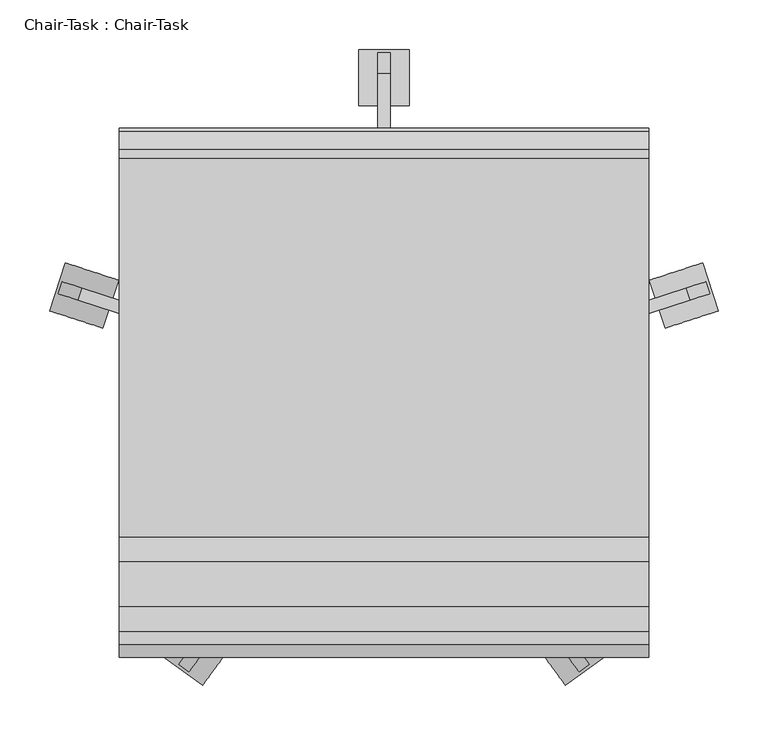
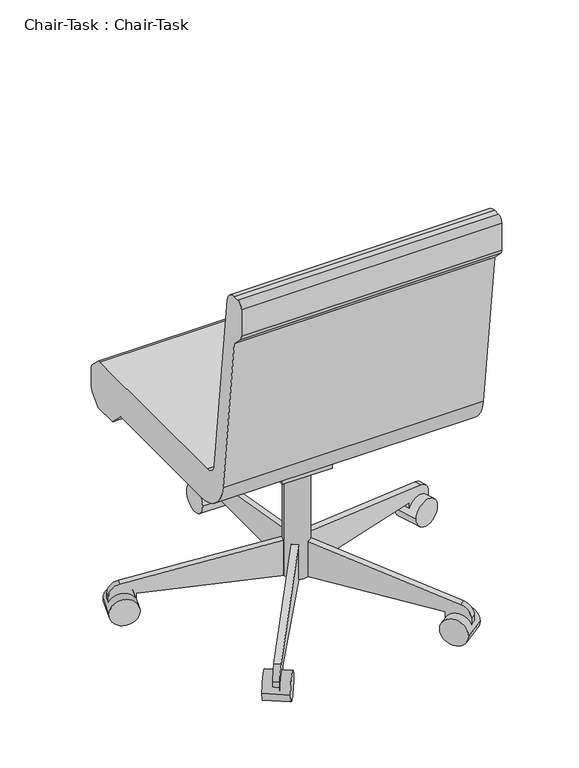
"""IFC4 building model written with IfcOpenShell, lengths in millimetres: furniture geometry, Chair-Task : Chair-Task."""

from ifc_helpers import new_model, si_unit, point, frame, frame_2d, origin, place, context, project, spatial, polyline, circle_curve, trimmed, segment, composite_curve, outline, extrude, source, transform, mapped, element, save


def chair_task_chair_task_b7f3823b(model_context):
    return source(origin(), model_context, "Body", "SweptSolid", [
        extrude(outline(composite_curve([segment(trimmed(circle_curve(frame_2d((140.9908197, 18.9459016)), 25.4), [point((115.5908197, 18.9459016))], [point((166.3908197, 18.9459016))], False, "CARTESIAN"), True, "CONTINUOUS"), segment(trimmed(circle_curve(frame_2d((140.9908197, 18.9459016)), 25.4), [point((166.3908197, 18.9459016))], [point((115.5908197, 18.9459016))], False, "CARTESIAN"), True, "CONTINUOUS")], self_intersect=False)), frame((0.0, 0.0, 53.5835944), z_axis=(0.0, 0.0, 1.0), x_axis=(1.0, 0.0, 0.0)), (0.0, 0.0, 1.0), 330.5914056),
        extrude(outline(composite_curve([segment(trimmed(circle_curve(frame_2d((0.0, -28.2002727)), 28.2002727), [point((0.0, -56.4005455))], [point((0.0, 0.0))], False, "CARTESIAN"), True, "CONTINUOUS"), segment(trimmed(circle_curve(frame_2d((0.0, -28.2002727)), 28.2002727), [point((0.0, 0.0))], [point((0.0, -56.4005455))], False, "CARTESIAN"), True, "CONTINUOUS")], self_intersect=False)), frame((477.6203484, 101.6163254, 28.1835944), z_axis=(-0.3090169943749423, 0.9510565162951553, 0.0), x_axis=(0.0, 0.0, 1.0)), (0.0, 0.0, 1.0), 50.8),
        extrude(outline(composite_curve([segment(polyline([(-25.4, 0.0), (0.0, 0.0), (0.0, -50.8), (-24.303053, -50.8)]), True, "CONTINUOUS"), segment(trimmed(circle_curve(frame_2d((-24.303053, -25.4)), 25.4), [point((-24.303053, -50.8))], [point((-49.3171699, -29.8106637))], False, "CARTESIAN"), True, "CONTINUOUS"), segment(polyline([(-49.3171699, -29.8106637), (-101.6, 266.7), (-101.6, 292.1), (-25.4, 292.1), (-25.4, 0.0)]), True, "CONTINUOUS")], self_intersect=False)), frame((420.756686, 103.1705568, 28.1835944), z_axis=(-0.3090169943749423, 0.9510565162951553, 0.0), x_axis=(0.0, 0.0, -1.0)), (0.0, 0.0, 1.0), 12.7),
        extrude(outline(composite_curve([segment(trimmed(circle_curve(frame_2d((0.0, -28.2002727)), 28.2002727), [point((0.0, -56.4005455))], [point((0.0, 0.0))], False, "CARTESIAN"), True, "CONTINUOUS"), segment(trimmed(circle_curve(frame_2d((0.0, -28.2002727)), 28.2002727), [point((0.0, 0.0))], [point((0.0, -56.4005455))], False, "CARTESIAN"), True, "CONTINUOUS")], self_intersect=False)), frame((323.63931, -275.6612394, 28.1835944), z_axis=(0.8090169943749499, 0.5877852522924699, 0.0), x_axis=(0.0, 0.0, 1.0)), (0.0, 0.0, 1.0), 50.8),
        extrude(outline(composite_curve([segment(polyline([(-25.4, 0.0), (0.0, 0.0), (0.0, -50.8), (-24.303053, -50.8)]), True, "CONTINUOUS"), segment(trimmed(circle_curve(frame_2d((-24.303053, -25.3999999)), 25.4), [point((-24.303053, -50.8))], [point((-49.3171699, -29.8106636))], False, "CARTESIAN"), True, "CONTINUOUS"), segment(polyline([(-49.3171699, -29.8106636), (-101.6, 266.7), (-101.6, 292.1), (-25.4, 292.1), (-25.4, 0.0)]), True, "CONTINUOUS")], self_intersect=False)), frame((307.545634, -221.1003988, 28.1835944), z_axis=(0.8090169943749499, 0.5877852522924699, 0.0), x_axis=(0.0, 0.0, -1.0)), (0.0, 0.0, 1.0), 12.7),
        extrude(outline(composite_curve([segment(trimmed(circle_curve(frame_2d((0.0, -28.2002727)), 28.2002727), [point((0.0, -56.4005455))], [point((0.0, 0.0))], False, "CARTESIAN"), True, "CONTINUOUS"), segment(trimmed(circle_curve(frame_2d((0.0, -28.2002727)), 28.2002727), [point((0.0, 0.0))], [point((0.0, -56.4005455))], False, "CARTESIAN"), True, "CONTINUOUS")], self_intersect=False)), frame((-41.6576707, -275.6612394, 28.1835944), z_axis=(-0.8090169943749458, 0.5877852522924754, 0.0), x_axis=(0.0, 0.0, -1.0)), (0.0, 0.0, 1.0), 50.8),
        extrude(outline(composite_curve([segment(polyline([(25.4, 0.0), (25.4, 292.1), (101.6, 292.1), (101.6, 266.7), (49.3171699, -29.8106637)]), True, "CONTINUOUS"), segment(trimmed(circle_curve(frame_2d((24.303053, -25.3999999)), 25.4), [point((49.3171699, -29.8106637))], [point((24.303053, -50.8))], False, "CARTESIAN"), True, "CONTINUOUS"), segment(polyline([(24.303053, -50.8), (0.0, -50.8), (0.0, 0.0), (25.4, 0.0)]), True, "CONTINUOUS")], self_intersect=False)), frame((-25.5639946, -221.1003988, 28.1835944), z_axis=(-0.8090169943749459, 0.5877852522924754, 0.0), x_axis=(0.0, 0.0, 1.0)), (0.0, 0.0, 1.0), 12.7),
        extrude(outline(composite_curve([segment(trimmed(circle_curve(frame_2d((0.0, -28.2002727)), 28.2002727), [point((0.0, -56.4005454))], [point((0.0, 0.0))], False, "CARTESIAN"), True, "CONTINUOUS"), segment(trimmed(circle_curve(frame_2d((0.0, -28.2002727)), 28.2002727), [point((0.0, 0.0))], [point((0.0, -56.4005454))], False, "CARTESIAN"), True, "CONTINUOUS")], self_intersect=False)), frame((-195.638709, 101.6163254, 28.1835944), z_axis=(0.3090169943749487, 0.9510565162951532, 0.0), x_axis=(0.0, 0.0, -1.0)), (0.0, 0.0, 1.0), 50.8),
        extrude(outline(composite_curve([segment(polyline([(25.4, 0.0), (25.4, 292.1000001), (101.6, 292.1000001), (101.6, 266.7), (49.3171699, -29.8106636)]), True, "CONTINUOUS"), segment(trimmed(circle_curve(frame_2d((24.303053, -25.4)), 25.4), [point((49.3171699, -29.8106636))], [point((24.303053, -50.8))], False, "CARTESIAN"), True, "CONTINUOUS"), segment(polyline([(24.303053, -50.8), (0.0, -50.8), (0.0, 0.0), (25.4, 0.0)]), True, "CONTINUOUS")], self_intersect=False)), frame((-138.7750467, 103.1705568, 28.1835944), z_axis=(0.3090169943749487, 0.9510565162951532, 0.0), x_axis=(0.0, 0.0, 1.0)), (0.0, 0.0, 1.0), 12.7),
        extrude(outline(composite_curve([segment(trimmed(circle_curve(frame_2d((336.4459016, 28.1835944)), 28.2002727), [point((308.2456289, 28.1835944))], [point((364.6461744, 28.1835944))], False, "CARTESIAN"), True, "CONTINUOUS"), segment(trimmed(circle_curve(frame_2d((336.4459016, 28.1835944)), 28.2002727), [point((364.6461744, 28.1835944))], [point((308.2456289, 28.1835944))], False, "CARTESIAN"), True, "CONTINUOUS")], self_intersect=False)), frame((115.5908197, 0.0, 0.0), z_axis=(1.0, 0.0, 0.0), x_axis=(0.0, 1.0, 0.0)), (0.0, 0.0, 1.0), 50.8),
        extrude(outline(composite_curve([segment(polyline([(311.0459016, 53.5835944), (18.9459016, 53.5835944), (18.9459016, 129.7835944), (44.3459016, 129.7835944), (340.8565654, 77.5007643)]), True, "CONTINUOUS"), segment(trimmed(circle_curve(frame_2d((336.4459016, 52.4866474)), 25.4), [point((340.8565654, 77.5007643))], [point((361.8459016, 52.4866474))], False, "CARTESIAN"), True, "CONTINUOUS"), segment(polyline([(361.8459016, 52.4866474), (361.8459016, 28.1835944), (311.0459016, 28.1835944), (311.0459016, 53.5835944)]), True, "CONTINUOUS")], self_intersect=False)), frame((134.6408197, 0.0, 0.0), z_axis=(1.0, 0.0, 0.0), x_axis=(0.0, 1.0, 0.0)), (0.0, 0.0, 1.0), 12.7),
        extrude(outline(polyline([(69.7459016, 383.7835944), (69.7459016, 371.0835944), (18.9459016, 283.0954134), (-19.1540984, 283.0954134), (-19.1540984, 383.7835944), (69.7459016, 383.7835944)])), frame((90.1908197, 0.0, 0.0), z_axis=(1.0, 0.0, 0.0), x_axis=(0.0, 1.0, 0.0)), (0.0, 0.0, 1.0), 101.6),
        extrude(outline(composite_curve([segment(polyline([(-126.2050455, 457.2), (255.0102301, 457.2)]), True, "CONTINUOUS"), segment(trimmed(circle_curve(frame_2d((255.0102301, 444.5)), 12.7), [point((255.0102301, 457.2))], [point((263.9604301, 453.510212))], False, "CARTESIAN"), True, "CONTINUOUS"), segment(polyline([(263.9604301, 453.510212), (281.8961016, 435.6939999)]), True, "CONTINUOUS"), segment(trimmed(circle_curve(frame_2d((272.9459016, 426.6837879)), 12.7), [point((281.8961016, 435.6939999))], [point((285.6459016, 426.6837879))], False, "CARTESIAN"), True, "CONTINUOUS"), segment(polyline([(285.6459016, 426.6837879), (285.6459016, 391.6405184)]), True, "CONTINUOUS"), segment(trimmed(circle_curve(frame_2d((260.2459016, 391.6405184)), 25.4), [point((285.6459016, 391.6405184))], [point((278.2663256, 373.7401184))], False, "CARTESIAN"), True, "CONTINUOUS"), segment(polyline([(278.2663256, 373.7401184), (260.2470284, 355.6), (209.4470284, 355.6), (181.0744602, 383.7835944), (-107.1089978, 383.7835944)]), True, "CONTINUOUS"), segment(trimmed(circle_curve(frame_2d((-107.1089978, 459.9835944)), 76.2), [point((-107.1089978, 383.7835944))], [point((-182.7870738, 451.0802913))], False, "CARTESIAN"), True, "CONTINUOUS"), segment(polyline([(-182.7870738, 451.0802913), (-222.3540984, 787.4), (-244.0343545, 809.0802561)]), True, "CONTINUOUS"), segment(trimmed(circle_curve(frame_2d((-235.0540984, 818.0605122)), 12.7), [point((-244.0343545, 809.0802561))], [point((-247.7540984, 818.0605122))], False, "CARTESIAN"), True, "CONTINUOUS"), segment(polyline([(-247.7540984, 818.0605122), (-247.7540984, 876.3)]), True, "CONTINUOUS"), segment(trimmed(circle_curve(frame_2d((-235.0540984, 876.3)), 12.7), [point((-247.7540984, 876.3))], [point((-235.0540984, 889.0))], False, "CARTESIAN"), True, "CONTINUOUS"), segment(polyline([(-235.0540984, 889.0), (-222.1789239, 889.0)]), True, "CONTINUOUS"), segment(trimmed(circle_curve(frame_2d((-222.1789239, 863.6)), 25.4), [point((-222.1789239, 889.0))], [point((-196.9528985, 866.5677677))], False, "CARTESIAN"), True, "CONTINUOUS"), segment(polyline([(-196.9528985, 866.5677677), (-151.4310708, 479.6322323)]), True, "CONTINUOUS"), segment(trimmed(circle_curve(frame_2d((-126.2050455, 482.6)), 25.4), [point((-151.4310708, 479.6322323))], [point((-126.2050455, 457.2))], True, "CARTESIAN"), True, "CONTINUOUS")], self_intersect=False)), frame((-125.7091803, 0.0, 0.0), z_axis=(1.0, 0.0, 0.0), x_axis=(0.0, 1.0, 0.0)), (0.0, 0.0, 1.0), 533.4),
    ])


if __name__ == "__main__":
    model = new_model("IFC4")
    model_context = context("Model", 3, world=origin())
    ifc_project = project(units=[si_unit("LENGTHUNIT", "METRE", prefix="MILLI")], contexts=[model_context])
    site = spatial("IfcSite", under=ifc_project)
    building = spatial("IfcBuilding", under=site)
    placement = place(None, origin())
    chair_task_chair_task_shape = chair_task_chair_task_b7f3823b(model_context)
    element("IfcFurniture", 1, ObjectType="Chair-Task : Chair-Task", at=placement, inside=building, context=model_context, shape_type="MappedRepresentation", body=[
        mapped(chair_task_chair_task_shape, transform((0.0, 0.0, 0.0), x_axis=(1.0, 0.0, 0.0), y_axis=(0.0, 1.0, 0.0), z_axis=(0.0, 0.0, 1.0))),
    ])
    save(model, "model.ifc")

# Revit data of these elements
# Type "Chair-Task : Chair-Task"
#   Assembly Code = "E2020200"
#   Base Material = Plastic, Opaque Black
#   Caster Material = Plastic, Opaque Black
#   Seat/Back Material = Textile - Slate Blue
#   Default Elevation = 0
# Element 1 (IfcFurniture, "Chair-Task : Chair-Task")
#   Materials on its faces: "Plastic, Opaque Black", "Textile - Slate Blue"
# Materials
#   "Plastic, Opaque Black": class "Plastic", colour RGB 0 0 0, transparency 0.7, Description = "Plastic, generic, opaque black", Cost = 0
#   "Textile - Slate Blue": class "Fabric", colour RGB 98 102 118, transparency 0
